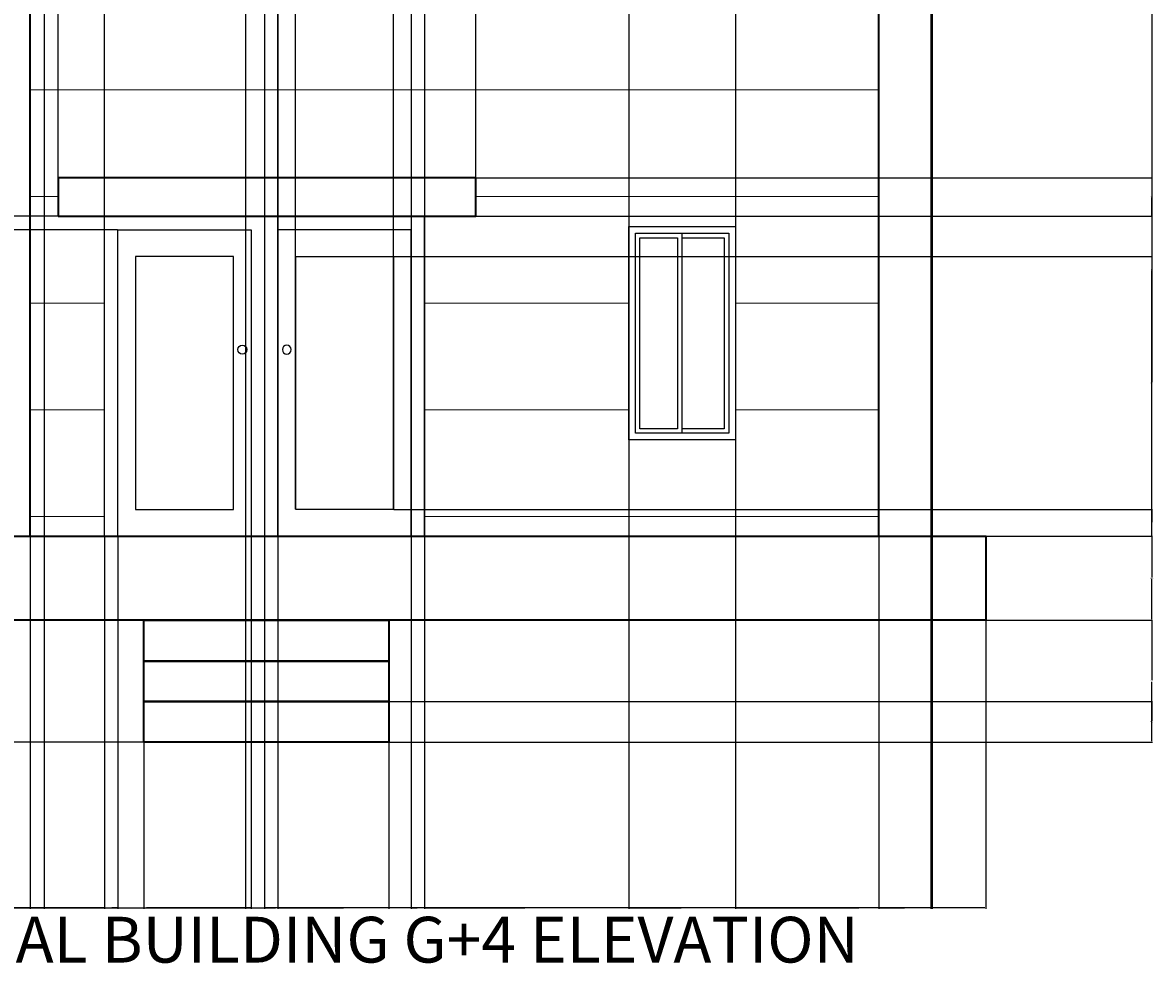
# Model space of a CAD drawing. Units: inches. Extents: x 10 to 404, y -77 to 696.
# Tile 2 of 5: x 149 to 404, y -77 to 135. Entities that reach past the tile are written whole.
import ezdxf

# ---------------------------------------------------------------- set-up
doc = ezdxf.new("R2010")
doc.units = ezdxf.units.IN
doc.header["$MEASUREMENT"] = 0
for name, color, linetype, lineweight in [('A-ANNO-DIMS', 2, 'Continuous', 18), ('A-ANNO-TEXT', 7, 'Continuous', 25), ('A-DOOR', 4, 'Continuous', 25), ('A-ELEV', 7, 'Continuous', 35), ('A-ELEV-PATT', 8, 'Continuous', 13), ('A-GLAZ', 4, 'Continuous', 25)]:
    doc.layers.add(name, color=color, linetype=linetype, lineweight=lineweight)
doc.styles.get("Standard").update_dxf_attribs({"font": 'arial.ttf'})
doc.dimstyles.get("Standard").update_dxf_attribs({"dimtxt": 0.18, "dimasz": 0.18, "dimexe": 0.18, "dimexo": 0.0625, "dimgap": 0.09, "dimtad": 0, "dimtih": 1, "dimtoh": 1, "dimdec": 4, "dimzin": 0, "dimdsep": 46, "dimtxsty": 'Standard', "dimcen": 0.09, "dimadec": 0, "dimazin": 0, "dimtfac": 1, "dimtdec": 4, "dimtofl": 0, "dimtmove": 0, "dimatfit": 3, "dimfxl": 1, "dimtolj": 1, "dimtzin": 0, "dimarcsym": 0})

# ---------------------------------------------------------------- blocks, each defined once
blk = doc.blocks.new('*U4')
blk.add_lwpolyline([(3.12, 0.01), (0.12, 0.01), (0.12, 72.01), (36.12, 72.01), (36.12, 0.01), (33.12, 0.01)])
for points in [[(33.12, 68.99), (33.12, 0.01), (3.12, 0.01), (3.12, 68.99)], [(29.12, 6.01), (29.12, 62.99), (7.12, 62.99), (7.12, 6.01)]]:
    blk.add_lwpolyline(points, close=True)
blk.add_circle((31.12, 42.01), 1)
blk = doc.blocks.new('*U5')
for p, q in [((1.5, 1.5), (1.5, 46.5)), ((1.5, 46.5), (12, 46.5)), ((12, 1.5), (12, 46.5)), ((12, 46.5), (22.5, 46.5)), ((22.5, 46.5), (22.5, 1.5)), ((12, 1.5), (1.5, 1.5)), ((22.5, 1.5), (12, 1.5))]:
    blk.add_line(p, q)
blk.add_lwpolyline([(0, 0), (0, 48), (24, 48), (24, 0)], close=True)
for points in [[(11, 45.5), (11, 2.5), (2.5, 2.5), (2.5, 45.5), (11, 45.5)], [(12, 45.5), (21.5, 45.5), (21.5, 2.5), (12, 2.5)]]:
    blk.add_lwpolyline(points)
blk = doc.blocks.new('*D9')
at = {"layer": 'A-ANNO-DIMS', "color": 0, "lineweight": -2, "transparency": 16777216}
for p, q in [((47.29, 0.6), (47.29, -64.31)), ((365.94, 0.6), (365.94, -64.31)), ((47.47, -64.13), (206.15, -64.13)), ((365.76, -64.13), (207.08, -64.13))]:
    blk.add_line(p, q, dxfattribs=at)
at = {"layer": 'A-ANNO-DIMS', "color": 0, "transparency": 16777216}
for points in [[(47.47, -64.1), (47.47, -64.16), (47.29, -64.13)], [(365.76, -64.1), (365.76, -64.16), (365.94, -64.13)]]:
    blk.add_solid(points, dxfattribs=at)
at = {"layer": 'Defpoints', "color": 0, "transparency": 16777216}
for p in [(47.29, 0.67), (365.94, 0.67), (365.94, -64.13)]:
    blk.add_point(p, dxfattribs=at)
at = {"layer": 'A-ANNO-DIMS', "color": 0, "transparency": 16777216, "insert": (206.61, -64.13), "char_height": 0.18, "attachment_point": 5}
blk.add_mtext('\\A1;318.65', dxfattribs=at)
blk = doc.blocks.new('*D10')
at = {"layer": 'A-ANNO-DIMS', "color": 0, "lineweight": -2, "transparency": 16777216}
for p, q in [((65.94, 657.96), (9.76, 657.96)), ((9.94, 657.78), (9.94, 315.77)), ((9.94, -26.6), (9.94, 315.41)), ((176.46, -26.78), (9.76, -26.78))]:
    blk.add_line(p, q, dxfattribs=at)
at = {"layer": 'A-ANNO-DIMS', "color": 0, "transparency": 16777216}
for points in [[(9.91, 657.78), (9.97, 657.78), (9.94, 657.96)], [(9.91, -26.6), (9.97, -26.6), (9.94, -26.78)]]:
    blk.add_solid(points, dxfattribs=at)
at = {"layer": 'Defpoints', "color": 0, "transparency": 16777216}
for p in [(9.94, 657.96), (66.01, 657.96), (176.53, -26.78)]:
    blk.add_point(p, dxfattribs=at)
at = {"layer": 'A-ANNO-DIMS', "color": 0, "transparency": 16777216, "insert": (9.94, 315.59), "char_height": 0.18, "attachment_point": 5}
blk.add_mtext('\\A1;684.7', dxfattribs=at)
blk = doc.blocks.new('*D13')
at = {"layer": 'A-ANNO-DIMS', "color": 0, "lineweight": -2, "transparency": 16777216}
for p, q in [((81.51, 19.49), (81.51, -64.31)), ((167.67, 19.49), (167.67, -64.31)), ((81.69, -64.13), (124.19, -64.13)), ((167.49, -64.13), (124.98, -64.13))]:
    blk.add_line(p, q, dxfattribs=at)
at = {"layer": 'A-ANNO-DIMS', "color": 0, "transparency": 16777216}
for points in [[(81.69, -64.1), (81.69, -64.16), (81.51, -64.13)], [(167.49, -64.1), (167.49, -64.16), (167.67, -64.13)]]:
    blk.add_solid(points, dxfattribs=at)
at = {"layer": 'Defpoints', "color": 0, "transparency": 16777216}
for p in [(81.51, 19.55), (167.67, 19.55), (167.67, -64.13)]:
    blk.add_point(p, dxfattribs=at)
at = {"layer": 'A-ANNO-DIMS', "color": 0, "transparency": 16777216, "insert": (124.59, -64.13), "char_height": 0.18, "attachment_point": 5}
blk.add_mtext('\\A1;86.16', dxfattribs=at)
blk = doc.blocks.new('*D14')
at = {"layer": 'A-ANNO-DIMS', "color": 0, "lineweight": -2, "transparency": 16777216}
for p, q in [((285.62, 41.17), (285.62, -64.31)), ((239.67, 19.49), (239.67, -64.31)), ((239.85, -64.13), (262.25, -64.13)), ((285.44, -64.13), (263.04, -64.13))]:
    blk.add_line(p, q, dxfattribs=at)
at = {"layer": 'A-ANNO-DIMS', "color": 0, "transparency": 16777216}
for points in [[(239.85, -64.1), (239.85, -64.16), (239.67, -64.13)], [(285.44, -64.1), (285.44, -64.16), (285.62, -64.13)]]:
    blk.add_solid(points, dxfattribs=at)
at = {"layer": 'Defpoints', "color": 0, "transparency": 16777216}
for p in [(285.62, 41.23), (239.67, 19.55), (285.62, -64.13)]:
    blk.add_point(p, dxfattribs=at)
at = {"layer": 'A-ANNO-DIMS', "color": 0, "transparency": 16777216, "insert": (262.64, -64.13), "char_height": 0.18, "attachment_point": 5}
blk.add_mtext('\\A1;45.95', dxfattribs=at)
blk = doc.blocks.new('*D15')
at = {"layer": 'A-ANNO-DIMS', "color": 0, "lineweight": -2, "transparency": 16777216}
for p, q in [((285.62, 41.17), (285.62, -64.31)), ((309.62, 41.17), (309.62, -64.31)), ((285.8, -64.13), (297.4, -64.13)), ((309.44, -64.13), (297.84, -64.13))]:
    blk.add_line(p, q, dxfattribs=at)
at = {"layer": 'A-ANNO-DIMS', "color": 0, "transparency": 16777216}
for points in [[(285.8, -64.1), (285.8, -64.16), (285.62, -64.13)], [(309.44, -64.1), (309.44, -64.16), (309.62, -64.13)]]:
    blk.add_solid(points, dxfattribs=at)
at = {"layer": 'Defpoints', "color": 0, "transparency": 16777216}
for p in [(285.62, 41.23), (309.62, 41.23), (309.62, -64.13)]:
    blk.add_point(p, dxfattribs=at)
at = {"layer": 'A-ANNO-DIMS', "color": 0, "transparency": 16777216, "insert": (297.62, -64.13), "char_height": 0.18, "attachment_point": 5}
blk.add_mtext('\\A1;24', dxfattribs=at)
blk = doc.blocks.new('*D16')
at = {"layer": 'A-ANNO-DIMS', "color": 0, "lineweight": -2, "transparency": 16777216}
for p, q in [((309.62, 41.17), (309.62, -64.31)), ((365.94, 0.6), (365.94, -64.31)), ((309.8, -64.13), (337.38, -64.13)), ((365.76, -64.13), (338.17, -64.13))]:
    blk.add_line(p, q, dxfattribs=at)
at = {"layer": 'A-ANNO-DIMS', "color": 0, "transparency": 16777216}
for points in [[(309.8, -64.1), (309.8, -64.16), (309.62, -64.13)], [(365.76, -64.1), (365.76, -64.16), (365.94, -64.13)]]:
    blk.add_solid(points, dxfattribs=at)
at = {"layer": 'Defpoints', "color": 0, "transparency": 16777216}
for p in [(309.62, 41.23), (365.94, 0.67), (365.94, -64.13)]:
    blk.add_point(p, dxfattribs=at)
at = {"layer": 'A-ANNO-DIMS', "color": 0, "transparency": 16777216, "insert": (337.78, -64.13), "char_height": 0.18, "attachment_point": 5}
blk.add_mtext('\\A1;56.32', dxfattribs=at)
blk = doc.blocks.new('*D23')
at = {"layer": 'A-ANNO-DIMS', "color": 0, "lineweight": -2, "transparency": 16777216}
for p, q in [((341.87, 355.52), (341.87, -64.31)), ((353.59, 355.52), (353.59, -64.31)), ((342.05, -64.13), (347.27, -64.13)), ((353.41, -64.13), (348.18, -64.13))]:
    blk.add_line(p, q, dxfattribs=at)
at = {"layer": 'A-ANNO-DIMS', "color": 0, "transparency": 16777216}
for points in [[(342.05, -64.1), (342.05, -64.16), (341.87, -64.13)], [(353.41, -64.1), (353.41, -64.16), (353.59, -64.13)]]:
    blk.add_solid(points, dxfattribs=at)
at = {"layer": 'Defpoints', "color": 0, "transparency": 16777216}
for p in [(341.87, 355.58), (353.59, 355.58), (353.59, -64.13)]:
    blk.add_point(p, dxfattribs=at)
at = {"layer": 'A-ANNO-DIMS', "color": 0, "transparency": 16777216, "insert": (347.73, -64.13), "char_height": 0.18, "attachment_point": 5}
blk.add_mtext('\\A1;11.723', dxfattribs=at)
blk = doc.blocks.new('*D24')
at = {"layer": 'A-ANNO-DIMS', "color": 0, "lineweight": -2, "transparency": 16777216}
for p, q in [((176.53, -26.84), (176.53, -64.31)), ((231.66, -26.84), (231.66, -64.31)), ((176.71, -64.13), (203.7, -64.13)), ((231.48, -64.13), (204.49, -64.13))]:
    blk.add_line(p, q, dxfattribs=at)
at = {"layer": 'A-ANNO-DIMS', "color": 0, "transparency": 16777216}
for points in [[(176.71, -64.1), (176.71, -64.16), (176.53, -64.13)], [(231.48, -64.1), (231.48, -64.16), (231.66, -64.13)]]:
    blk.add_solid(points, dxfattribs=at)
at = {"layer": 'Defpoints', "color": 0, "transparency": 16777216}
for p in [(176.53, -26.78), (231.66, -26.78), (231.66, -64.13)]:
    blk.add_point(p, dxfattribs=at)
at = {"layer": 'A-ANNO-DIMS', "color": 0, "transparency": 16777216, "insert": (204.09, -64.13), "char_height": 0.18, "attachment_point": 5}
blk.add_mtext('\\A1;55.13', dxfattribs=at)
blk = doc.blocks.new('*D25')
at = {"layer": 'A-ANNO-DIMS', "color": 0, "lineweight": -2, "transparency": 16777216}
for p, q in [((231.72, 0.67), (403.47, 0.67)), ((403.29, 0.49), (403.29, -12.88)), ((403.29, -26.6), (403.29, -13.24)), ((231.72, -26.78), (403.47, -26.78))]:
    blk.add_line(p, q, dxfattribs=at)
at = {"layer": 'A-ANNO-DIMS', "color": 0, "transparency": 16777216}
for points in [[(403.26, 0.49), (403.32, 0.49), (403.29, 0.67)], [(403.26, -26.6), (403.32, -26.6), (403.29, -26.78)]]:
    blk.add_solid(points, dxfattribs=at)
at = {"layer": 'Defpoints', "color": 0, "transparency": 16777216}
for p in [(231.66, 0.67), (231.66, -26.78), (403.29, -26.78)]:
    blk.add_point(p, dxfattribs=at)
at = {"layer": 'A-ANNO-DIMS', "color": 0, "transparency": 16777216, "insert": (403.29, -13.06), "char_height": 0.18, "attachment_point": 5}
blk.add_mtext('\\A1;27.45', dxfattribs=at)
blk = doc.blocks.new('*D26')
at = {"layer": 'A-ANNO-DIMS', "color": 0, "lineweight": -2, "transparency": 16777216}
for p, q in [((231.72, -17.67), (403.47, -17.67)), ((403.29, -17.85), (403.29, -22.04)), ((403.29, -26.6), (403.29, -22.41)), ((231.72, -26.78), (403.47, -26.78))]:
    blk.add_line(p, q, dxfattribs=at)
at = {"layer": 'A-ANNO-DIMS', "color": 0, "transparency": 16777216}
for points in [[(403.26, -17.85), (403.32, -17.85), (403.29, -17.67)], [(403.26, -26.6), (403.32, -26.6), (403.29, -26.78)]]:
    blk.add_solid(points, dxfattribs=at)
at = {"layer": 'Defpoints', "color": 0, "transparency": 16777216}
for p in [(231.66, -17.67), (231.66, -26.78), (403.29, -26.78)]:
    blk.add_point(p, dxfattribs=at)
at = {"layer": 'A-ANNO-DIMS', "color": 0, "transparency": 16777216, "insert": (403.29, -22.22), "char_height": 0.18, "attachment_point": 5}
blk.add_mtext('\\A1;9.115', dxfattribs=at)
blk = doc.blocks.new('*D27')
at = {"layer": 'A-ANNO-DIMS', "color": 0, "lineweight": -2, "transparency": 16777216}
for p, q in [((366, 19.55), (403.47, 19.55)), ((403.29, 19.37), (403.29, 10.29)), ((403.29, 0.85), (403.29, 9.93)), ((366, 0.67), (403.47, 0.67))]:
    blk.add_line(p, q, dxfattribs=at)
at = {"layer": 'A-ANNO-DIMS', "color": 0, "transparency": 16777216}
for points in [[(403.26, 19.37), (403.32, 19.37), (403.29, 19.55)], [(403.26, 0.85), (403.32, 0.85), (403.29, 0.67)]]:
    blk.add_solid(points, dxfattribs=at)
at = {"layer": 'Defpoints', "color": 0, "transparency": 16777216}
for p in [(365.94, 19.55), (403.29, 19.55), (365.94, 0.67)]:
    blk.add_point(p, dxfattribs=at)
at = {"layer": 'A-ANNO-DIMS', "color": 0, "transparency": 16777216, "insert": (403.29, 10.11), "char_height": 0.18, "attachment_point": 5}
blk.add_mtext('\\A1;18.887', dxfattribs=at)
blk = doc.blocks.new('*D28')
at = {"layer": 'A-ANNO-DIMS', "color": 0, "lineweight": -2, "transparency": 16777216}
for p, q in [((341.93, 139.55), (403.47, 139.55)), ((403.29, 139.37), (403.29, 79.74)), ((403.29, 19.73), (403.29, 79.37)), ((341.93, 19.55), (403.47, 19.55))]:
    blk.add_line(p, q, dxfattribs=at)
at = {"layer": 'A-ANNO-DIMS', "color": 0, "transparency": 16777216}
for points in [[(403.26, 139.37), (403.32, 139.37), (403.29, 139.55)], [(403.26, 19.73), (403.32, 19.73), (403.29, 19.55)]]:
    blk.add_solid(points, dxfattribs=at)
at = {"layer": 'Defpoints', "color": 0, "transparency": 16777216}
for p in [(341.87, 139.55), (403.29, 139.55), (341.87, 19.55)]:
    blk.add_point(p, dxfattribs=at)
at = {"layer": 'A-ANNO-DIMS', "color": 0, "transparency": 16777216, "insert": (403.29, 79.55), "char_height": 0.18, "attachment_point": 5}
blk.add_mtext('\\A1;120', dxfattribs=at)
blk = doc.blocks.new('*D39')
at = {"layer": 'A-ANNO-DIMS', "color": 0, "lineweight": -2, "transparency": 16777216}
for p, q in [((341.87, 259.49), (341.87, -64.31)), ((353.87, 259.49), (353.87, -64.31)), ((342.05, -64.13), (347.66, -64.13)), ((353.69, -64.13), (348.08, -64.13))]:
    blk.add_line(p, q, dxfattribs=at)
at = {"layer": 'A-ANNO-DIMS', "color": 0, "transparency": 16777216}
for points in [[(342.05, -64.1), (342.05, -64.16), (341.87, -64.13)], [(353.69, -64.1), (353.69, -64.16), (353.87, -64.13)]]:
    blk.add_solid(points, dxfattribs=at)
at = {"layer": 'Defpoints', "color": 0, "transparency": 16777216}
for p in [(341.87, 259.55), (353.87, 259.55), (353.87, -64.13)]:
    blk.add_point(p, dxfattribs=at)
at = {"layer": 'A-ANNO-DIMS', "color": 0, "transparency": 16777216, "insert": (347.87, -64.13), "char_height": 0.18, "attachment_point": 5}
blk.add_mtext('\\A1;12', dxfattribs=at)
blk = doc.blocks.new('*D42')
at = {"layer": 'A-ANNO-DIMS', "color": 0, "lineweight": -2, "transparency": 16777216}
for p, q in [((150.93, 259.49), (150.93, -64.31)), ((154.06, 142.19), (154.06, -64.31)), ((151.11, -64.13), (152.17, -64.13)), ((153.88, -64.13), (152.82, -64.13))]:
    blk.add_line(p, q, dxfattribs=at)
at = {"layer": 'A-ANNO-DIMS', "color": 0, "transparency": 16777216}
for points in [[(151.11, -64.1), (151.11, -64.16), (150.93, -64.13)], [(153.88, -64.1), (153.88, -64.16), (154.06, -64.13)]]:
    blk.add_solid(points, dxfattribs=at)
at = {"layer": 'Defpoints', "color": 0, "transparency": 16777216}
for p in [(150.93, 259.55), (154.06, 142.25), (154.06, -64.13)]:
    blk.add_point(p, dxfattribs=at)
at = {"layer": 'A-ANNO-DIMS', "color": 0, "transparency": 16777216, "insert": (152.5, -64.13), "char_height": 0.18, "attachment_point": 5}
blk.add_mtext('\\A1;3.13', dxfattribs=at)
blk = doc.blocks.new('*D43')
at = {"layer": 'A-ANNO-DIMS', "color": 0, "lineweight": -2, "transparency": 16777216}
for p, q in [((154.06, 142.19), (154.06, -64.31)), ((199.39, 142.19), (199.39, -64.31)), ((154.24, -64.13), (176.33, -64.13)), ((199.21, -64.13), (177.13, -64.13))]:
    blk.add_line(p, q, dxfattribs=at)
at = {"layer": 'A-ANNO-DIMS', "color": 0, "transparency": 16777216}
for points in [[(154.24, -64.1), (154.24, -64.16), (154.06, -64.13)], [(199.21, -64.1), (199.21, -64.16), (199.39, -64.13)]]:
    blk.add_solid(points, dxfattribs=at)
at = {"layer": 'Defpoints', "color": 0, "transparency": 16777216}
for p in [(154.06, 142.25), (199.39, 142.25), (199.39, -64.13)]:
    blk.add_point(p, dxfattribs=at)
at = {"layer": 'A-ANNO-DIMS', "color": 0, "transparency": 16777216, "insert": (176.73, -64.13), "char_height": 0.18, "attachment_point": 5}
blk.add_mtext('\\A1;45.33', dxfattribs=at)
blk = doc.blocks.new('*D48')
at = {"layer": 'A-ANNO-DIMS', "color": 0, "lineweight": -2, "transparency": 16777216}
for p, q in [((285.62, 521.17), (285.62, -64.31)), ((239.67, 499.54), (239.67, -64.31)), ((239.85, -64.13), (262.25, -64.13)), ((285.44, -64.13), (263.04, -64.13))]:
    blk.add_line(p, q, dxfattribs=at)
at = {"layer": 'A-ANNO-DIMS', "color": 0, "transparency": 16777216}
for points in [[(239.85, -64.1), (239.85, -64.16), (239.67, -64.13)], [(285.44, -64.1), (285.44, -64.16), (285.62, -64.13)]]:
    blk.add_solid(points, dxfattribs=at)
at = {"layer": 'Defpoints', "color": 0, "transparency": 16777216}
for p in [(285.62, 521.23), (239.67, 499.6), (285.62, -64.13)]:
    blk.add_point(p, dxfattribs=at)
at = {"layer": 'A-ANNO-DIMS', "color": 0, "transparency": 16777216, "insert": (262.64, -64.13), "char_height": 0.18, "attachment_point": 5}
blk.add_mtext('\\A1;45.95', dxfattribs=at)
blk = doc.blocks.new('*D49')
at = {"layer": 'A-ANNO-DIMS', "color": 0, "lineweight": -2, "transparency": 16777216}
for p, q in [((285.62, 521.17), (285.62, -64.31)), ((309.62, 521.17), (309.62, -64.31)), ((285.8, -64.13), (297.4, -64.13)), ((309.44, -64.13), (297.84, -64.13))]:
    blk.add_line(p, q, dxfattribs=at)
at = {"layer": 'A-ANNO-DIMS', "color": 0, "transparency": 16777216}
for points in [[(285.8, -64.1), (285.8, -64.16), (285.62, -64.13)], [(309.44, -64.1), (309.44, -64.16), (309.62, -64.13)]]:
    blk.add_solid(points, dxfattribs=at)
at = {"layer": 'Defpoints', "color": 0, "transparency": 16777216}
for p in [(285.62, 521.23), (309.62, 521.23), (309.62, -64.13)]:
    blk.add_point(p, dxfattribs=at)
at = {"layer": 'A-ANNO-DIMS', "color": 0, "transparency": 16777216, "insert": (297.62, -64.13), "char_height": 0.18, "attachment_point": 5}
blk.add_mtext('\\A1;24', dxfattribs=at)
blk = doc.blocks.new('*D50')
at = {"layer": 'A-ANNO-DIMS', "color": 0, "lineweight": -2, "transparency": 16777216}
for p, q in [((157.2, 100.31), (157.2, 695.87)), ((157.38, 695.69), (161.98, 695.69)), ((167.49, 695.69), (162.89, 695.69)), ((167.67, 91.62), (167.67, 695.87))]:
    blk.add_line(p, q, dxfattribs=at)
at = {"layer": 'A-ANNO-DIMS', "color": 0, "transparency": 16777216}
for points in [[(157.38, 695.72), (157.38, 695.66), (157.2, 695.69)], [(167.49, 695.72), (167.49, 695.66), (167.67, 695.69)]]:
    blk.add_solid(points, dxfattribs=at)
at = {"layer": 'Defpoints', "color": 0, "transparency": 16777216}
for p in [(167.67, 695.69), (157.2, 100.24), (167.67, 91.55)]:
    blk.add_point(p, dxfattribs=at)
at = {"layer": 'A-ANNO-DIMS', "color": 0, "transparency": 16777216, "insert": (162.43, 695.69), "char_height": 0.18, "attachment_point": 5}
blk.add_mtext('\\A1;10.469', dxfattribs=at)
blk = doc.blocks.new('*D51')
at = {"layer": 'A-ANNO-DIMS', "color": 0, "lineweight": -2, "transparency": 16777216}
for p, q in [((167.67, 91.62), (167.67, 695.87)), ((167.85, 695.69), (209.06, 695.69)), ((251.06, 695.69), (209.85, 695.69)), ((251.24, 100.31), (251.24, 695.87))]:
    blk.add_line(p, q, dxfattribs=at)
at = {"layer": 'A-ANNO-DIMS', "color": 0, "transparency": 16777216}
for points in [[(167.85, 695.72), (167.85, 695.66), (167.67, 695.69)], [(251.06, 695.72), (251.06, 695.66), (251.24, 695.69)]]:
    blk.add_solid(points, dxfattribs=at)
at = {"layer": 'Defpoints', "color": 0, "transparency": 16777216}
for p in [(251.24, 695.69), (251.24, 100.24), (167.67, 91.55)]:
    blk.add_point(p, dxfattribs=at)
at = {"layer": 'A-ANNO-DIMS', "color": 0, "transparency": 16777216, "insert": (209.45, 695.69), "char_height": 0.18, "attachment_point": 5}
blk.add_mtext('\\A1;83.57', dxfattribs=at)
blk = doc.blocks.new('*D52')
at = {"layer": 'A-ANNO-DIMS', "color": 0, "lineweight": -2, "transparency": 16777216}
for p, q in [((251.3, 100.24), (403.47, 100.24)), ((403.29, 100.06), (403.29, 96.08)), ((403.29, 91.73), (403.29, 95.72)), ((251.3, 91.55), (403.47, 91.55))]:
    blk.add_line(p, q, dxfattribs=at)
at = {"layer": 'A-ANNO-DIMS', "color": 0, "transparency": 16777216}
for points in [[(403.26, 100.06), (403.32, 100.06), (403.29, 100.24)], [(403.26, 91.73), (403.32, 91.73), (403.29, 91.55)]]:
    blk.add_solid(points, dxfattribs=at)
at = {"layer": 'Defpoints', "color": 0, "transparency": 16777216}
for p in [(251.24, 100.24), (403.29, 100.24), (251.24, 91.55)]:
    blk.add_point(p, dxfattribs=at)
at = {"layer": 'A-ANNO-DIMS', "color": 0, "transparency": 16777216, "insert": (403.29, 95.9), "char_height": 0.18, "attachment_point": 5}
blk.add_mtext('\\A1;8.69', dxfattribs=at)
blk = doc.blocks.new('*D53')
at = {"layer": 'A-ANNO-DIMS', "color": 0, "lineweight": -2, "transparency": 16777216}
for p, q in [((251.3, 91.55), (403.47, 91.55)), ((403.29, 91.37), (403.29, 55.73)), ((403.29, 19.73), (403.29, 55.37)), ((239.73, 19.55), (403.47, 19.55))]:
    blk.add_line(p, q, dxfattribs=at)
at = {"layer": 'A-ANNO-DIMS', "color": 0, "transparency": 16777216}
for points in [[(403.26, 91.37), (403.32, 91.37), (403.29, 91.55)], [(403.26, 19.73), (403.32, 19.73), (403.29, 19.55)]]:
    blk.add_solid(points, dxfattribs=at)
at = {"layer": 'Defpoints', "color": 0, "transparency": 16777216}
for p in [(251.24, 91.55), (403.29, 91.55), (239.67, 19.55)]:
    blk.add_point(p, dxfattribs=at)
at = {"layer": 'A-ANNO-DIMS', "color": 0, "transparency": 16777216, "insert": (403.29, 55.55), "char_height": 0.18, "attachment_point": 5}
blk.add_mtext('\\A1;72', dxfattribs=at)
blk = doc.blocks.new('*D54')
at = {"layer": 'A-ANNO-DIMS', "color": 0, "lineweight": -2, "transparency": 16777216}
for p, q in [((167.6, 91.55), (9.76, 91.55)), ((9.94, 91.37), (9.94, 55.73)), ((9.94, 19.73), (9.94, 55.37)), ((167.6, 19.55), (9.76, 19.55))]:
    blk.add_line(p, q, dxfattribs=at)
at = {"layer": 'A-ANNO-DIMS', "color": 0, "transparency": 16777216}
for points in [[(9.91, 91.37), (9.97, 91.37), (9.94, 91.55)], [(9.91, 19.73), (9.97, 19.73), (9.94, 19.55)]]:
    blk.add_solid(points, dxfattribs=at)
at = {"layer": 'Defpoints', "color": 0, "transparency": 16777216}
for p in [(9.94, 91.55), (167.67, 91.55), (167.67, 19.55)]:
    blk.add_point(p, dxfattribs=at)
at = {"layer": 'A-ANNO-DIMS', "color": 0, "transparency": 16777216, "insert": (9.94, 55.55), "char_height": 0.18, "attachment_point": 5}
blk.add_mtext('\\A1;72', dxfattribs=at)
blk = doc.blocks.new('*D55')
at = {"layer": 'A-ANNO-DIMS', "color": 0, "lineweight": -2, "transparency": 16777216}
for p, q in [((170.6, 88.53), (9.76, 88.53)), ((9.94, 88.35), (9.94, 54.22)), ((9.94, 19.73), (9.94, 53.86)), ((170.6, 19.55), (9.76, 19.55))]:
    blk.add_line(p, q, dxfattribs=at)
at = {"layer": 'A-ANNO-DIMS', "color": 0, "transparency": 16777216}
for points in [[(9.91, 88.35), (9.97, 88.35), (9.94, 88.53)], [(9.91, 19.73), (9.97, 19.73), (9.94, 19.55)]]:
    blk.add_solid(points, dxfattribs=at)
at = {"layer": 'Defpoints', "color": 0, "transparency": 16777216}
for p in [(9.94, 88.53), (170.67, 88.53), (170.67, 19.55)]:
    blk.add_point(p, dxfattribs=at)
at = {"layer": 'A-ANNO-DIMS', "color": 0, "transparency": 16777216, "insert": (9.94, 54.04), "char_height": 0.18, "attachment_point": 5}
blk.add_mtext('\\A1;68.98', dxfattribs=at)
blk = doc.blocks.new('*D56')
at = {"layer": 'A-ANNO-DIMS', "color": 0, "lineweight": -2, "transparency": 16777216}
for p, q in [((167.67, 19.49), (167.67, -64.31)), ((170.67, 19.49), (170.67, -64.31)), ((167.85, -64.13), (169.02, -64.13)), ((170.49, -64.13), (169.32, -64.13))]:
    blk.add_line(p, q, dxfattribs=at)
at = {"layer": 'A-ANNO-DIMS', "color": 0, "transparency": 16777216}
for points in [[(167.85, -64.1), (167.85, -64.16), (167.67, -64.13)], [(170.49, -64.1), (170.49, -64.16), (170.67, -64.13)]]:
    blk.add_solid(points, dxfattribs=at)
at = {"layer": 'Defpoints', "color": 0, "transparency": 16777216}
for p in [(167.67, 19.55), (170.67, 19.55), (170.67, -64.13)]:
    blk.add_point(p, dxfattribs=at)
at = {"layer": 'A-ANNO-DIMS', "color": 0, "transparency": 16777216, "insert": (169.17, -64.13), "char_height": 0.18, "attachment_point": 5}
blk.add_mtext('\\A1;3', dxfattribs=at)
blk = doc.blocks.new('*D57')
at = {"layer": 'A-ANNO-DIMS', "color": 0, "lineweight": -2, "transparency": 16777216}
for p, q in [((170.67, 19.49), (170.67, -64.31)), ((200.67, 19.49), (200.67, -64.31)), ((170.85, -64.13), (185.45, -64.13)), ((200.49, -64.13), (185.89, -64.13))]:
    blk.add_line(p, q, dxfattribs=at)
at = {"layer": 'A-ANNO-DIMS', "color": 0, "transparency": 16777216}
for points in [[(170.85, -64.1), (170.85, -64.16), (170.67, -64.13)], [(200.49, -64.1), (200.49, -64.16), (200.67, -64.13)]]:
    blk.add_solid(points, dxfattribs=at)
at = {"layer": 'Defpoints', "color": 0, "transparency": 16777216}
for p in [(170.67, 19.55), (200.67, 19.55), (200.67, -64.13)]:
    blk.add_point(p, dxfattribs=at)
at = {"layer": 'A-ANNO-DIMS', "color": 0, "transparency": 16777216, "insert": (185.67, -64.13), "char_height": 0.18, "attachment_point": 5}
blk.add_mtext('\\A1;30', dxfattribs=at)
blk = doc.blocks.new('*D58')
at = {"layer": 'A-ANNO-DIMS', "color": 0, "lineweight": -2, "transparency": 16777216}
for p, q in [((200.67, 19.49), (200.67, -64.31)), ((206.67, 19.49), (206.67, -64.31)), ((200.85, -64.13), (203.52, -64.13)), ((206.49, -64.13), (203.82, -64.13))]:
    blk.add_line(p, q, dxfattribs=at)
at = {"layer": 'A-ANNO-DIMS', "color": 0, "transparency": 16777216}
for points in [[(200.85, -64.1), (200.85, -64.16), (200.67, -64.13)], [(206.49, -64.1), (206.49, -64.16), (206.67, -64.13)]]:
    blk.add_solid(points, dxfattribs=at)
at = {"layer": 'Defpoints', "color": 0, "transparency": 16777216}
for p in [(200.67, 19.55), (206.67, 19.55), (206.67, -64.13)]:
    blk.add_point(p, dxfattribs=at)
at = {"layer": 'A-ANNO-DIMS', "color": 0, "transparency": 16777216, "insert": (203.67, -64.13), "char_height": 0.18, "attachment_point": 5}
blk.add_mtext('\\A1;6', dxfattribs=at)
blk = doc.blocks.new('*D59')
at = {"layer": 'A-ANNO-DIMS', "color": 0, "lineweight": -2, "transparency": 16777216}
for p, q in [((206.67, 19.49), (206.67, -64.31)), ((236.67, 19.49), (236.67, -64.31)), ((206.85, -64.13), (221.45, -64.13)), ((236.49, -64.13), (221.89, -64.13))]:
    blk.add_line(p, q, dxfattribs=at)
at = {"layer": 'A-ANNO-DIMS', "color": 0, "transparency": 16777216}
for points in [[(206.85, -64.1), (206.85, -64.16), (206.67, -64.13)], [(236.49, -64.1), (236.49, -64.16), (236.67, -64.13)]]:
    blk.add_solid(points, dxfattribs=at)
at = {"layer": 'Defpoints', "color": 0, "transparency": 16777216}
for p in [(206.67, 19.55), (236.67, 19.55), (236.67, -64.13)]:
    blk.add_point(p, dxfattribs=at)
at = {"layer": 'A-ANNO-DIMS', "color": 0, "transparency": 16777216, "insert": (221.67, -64.13), "char_height": 0.18, "attachment_point": 5}
blk.add_mtext('\\A1;30', dxfattribs=at)
blk = doc.blocks.new('*D60')
at = {"layer": 'A-ANNO-DIMS', "color": 0, "lineweight": -2, "transparency": 16777216}
for p, q in [((236.67, 19.49), (236.67, -64.31)), ((239.67, 19.49), (239.67, -64.31)), ((236.85, -64.13), (238.02, -64.13)), ((239.49, -64.13), (238.32, -64.13))]:
    blk.add_line(p, q, dxfattribs=at)
at = {"layer": 'A-ANNO-DIMS', "color": 0, "transparency": 16777216}
for points in [[(236.85, -64.1), (236.85, -64.16), (236.67, -64.13)], [(239.49, -64.1), (239.49, -64.16), (239.67, -64.13)]]:
    blk.add_solid(points, dxfattribs=at)
at = {"layer": 'Defpoints', "color": 0, "transparency": 16777216}
for p in [(236.67, 19.55), (239.67, 19.55), (239.67, -64.13)]:
    blk.add_point(p, dxfattribs=at)
at = {"layer": 'A-ANNO-DIMS', "color": 0, "transparency": 16777216, "insert": (238.17, -64.13), "char_height": 0.18, "attachment_point": 5}
blk.add_mtext('\\A1;3', dxfattribs=at)
blk = doc.blocks.new('*D61')
at = {"layer": 'A-ANNO-DIMS', "color": 0, "lineweight": -2, "transparency": 16777216}
for p, q in [((206.67, 19.62), (206.67, 695.87)), ((206.85, 695.69), (208.51, 695.69)), ((210.49, 695.69), (208.82, 695.69)), ((210.67, 25.62), (210.67, 695.87))]:
    blk.add_line(p, q, dxfattribs=at)
at = {"layer": 'A-ANNO-DIMS', "color": 0, "transparency": 16777216}
for points in [[(206.85, 695.72), (206.85, 695.66), (206.67, 695.69)], [(210.49, 695.72), (210.49, 695.66), (210.67, 695.69)]]:
    blk.add_solid(points, dxfattribs=at)
at = {"layer": 'Defpoints', "color": 0, "transparency": 16777216}
for p in [(210.67, 695.69), (210.67, 25.55), (206.67, 19.55)]:
    blk.add_point(p, dxfattribs=at)
at = {"layer": 'A-ANNO-DIMS', "color": 0, "transparency": 16777216, "insert": (208.67, 695.69), "char_height": 0.18, "attachment_point": 5}
blk.add_mtext('\\A1;4', dxfattribs=at)
blk = doc.blocks.new('*D62')
at = {"layer": 'A-ANNO-DIMS', "color": 0, "lineweight": -2, "transparency": 16777216}
for p, q in [((210.67, 25.62), (210.67, 695.87)), ((210.85, 695.69), (221.45, 695.69)), ((232.49, 695.69), (221.89, 695.69)), ((232.67, 25.62), (232.67, 695.87))]:
    blk.add_line(p, q, dxfattribs=at)
at = {"layer": 'A-ANNO-DIMS', "color": 0, "transparency": 16777216}
for points in [[(210.85, 695.72), (210.85, 695.66), (210.67, 695.69)], [(232.49, 695.72), (232.49, 695.66), (232.67, 695.69)]]:
    blk.add_solid(points, dxfattribs=at)
at = {"layer": 'Defpoints', "color": 0, "transparency": 16777216}
for p in [(232.67, 695.69), (210.67, 25.55), (232.67, 25.55)]:
    blk.add_point(p, dxfattribs=at)
at = {"layer": 'A-ANNO-DIMS', "color": 0, "transparency": 16777216, "insert": (221.67, 695.69), "char_height": 0.18, "attachment_point": 5}
blk.add_mtext('\\A1;22', dxfattribs=at)
blk = doc.blocks.new('*D63')
at = {"layer": 'A-ANNO-DIMS', "color": 0, "lineweight": -2, "transparency": 16777216}
for p, q in [((232.73, 25.55), (403.47, 25.55)), ((403.29, 25.37), (403.29, 22.74)), ((403.29, 19.73), (403.29, 22.37)), ((236.73, 19.55), (403.47, 19.55))]:
    blk.add_line(p, q, dxfattribs=at)
at = {"layer": 'A-ANNO-DIMS', "color": 0, "transparency": 16777216}
for points in [[(403.26, 25.37), (403.32, 25.37), (403.29, 25.55)], [(403.26, 19.73), (403.32, 19.73), (403.29, 19.55)]]:
    blk.add_solid(points, dxfattribs=at)
at = {"layer": 'Defpoints', "color": 0, "transparency": 16777216}
for p in [(232.67, 25.55), (403.29, 25.55), (236.67, 19.55)]:
    blk.add_point(p, dxfattribs=at)
at = {"layer": 'A-ANNO-DIMS', "color": 0, "transparency": 16777216, "insert": (403.29, 22.55), "char_height": 0.18, "attachment_point": 5}
blk.add_mtext('\\A1;6', dxfattribs=at)
blk = doc.blocks.new('*D64')
at = {"layer": 'A-ANNO-DIMS', "color": 0, "lineweight": -2, "transparency": 16777216}
for p, q in [((232.73, 82.53), (403.47, 82.53)), ((403.29, 82.35), (403.29, 54.22)), ((403.29, 25.73), (403.29, 53.86)), ((232.73, 25.55), (403.47, 25.55))]:
    blk.add_line(p, q, dxfattribs=at)
at = {"layer": 'A-ANNO-DIMS', "color": 0, "transparency": 16777216}
for points in [[(403.26, 82.35), (403.32, 82.35), (403.29, 82.53)], [(403.26, 25.73), (403.32, 25.73), (403.29, 25.55)]]:
    blk.add_solid(points, dxfattribs=at)
at = {"layer": 'Defpoints', "color": 0, "transparency": 16777216}
for p in [(232.67, 82.53), (403.29, 82.53), (232.67, 25.55)]:
    blk.add_point(p, dxfattribs=at)
at = {"layer": 'A-ANNO-DIMS', "color": 0, "transparency": 16777216, "insert": (403.29, 54.04), "char_height": 0.18, "attachment_point": 5}
blk.add_mtext('\\A1;56.98', dxfattribs=at)
blk = doc.blocks.new('*D66')
at = {"layer": 'A-ANNO-DIMS', "color": 0, "lineweight": -2, "transparency": 16777216}
for p, q in [((203.67, 499.54), (203.67, -64.31)), ((206.67, 499.54), (206.67, -64.31)), ((203.85, -64.13), (205.02, -64.13)), ((206.49, -64.13), (205.32, -64.13))]:
    blk.add_line(p, q, dxfattribs=at)
at = {"layer": 'A-ANNO-DIMS', "color": 0, "transparency": 16777216}
for points in [[(203.85, -64.1), (203.85, -64.16), (203.67, -64.13)], [(206.49, -64.1), (206.49, -64.16), (206.67, -64.13)]]:
    blk.add_solid(points, dxfattribs=at)
at = {"layer": 'Defpoints', "color": 0, "transparency": 16777216}
for p in [(203.67, 499.6), (206.67, 499.6), (206.67, -64.13)]:
    blk.add_point(p, dxfattribs=at)
at = {"layer": 'A-ANNO-DIMS', "color": 0, "transparency": 16777216, "insert": (205.17, -64.13), "char_height": 0.18, "attachment_point": 5}
blk.add_mtext('\\A1;3', dxfattribs=at)
blk = doc.blocks.new('*D67')
at = {"layer": 'A-ANNO-DIMS', "color": 0, "lineweight": -2, "transparency": 16777216}
for p, q in [((206.67, 499.54), (206.67, -64.31)), ((236.67, 499.54), (236.67, -64.31)), ((206.85, -64.13), (221.45, -64.13)), ((236.49, -64.13), (221.89, -64.13))]:
    blk.add_line(p, q, dxfattribs=at)
at = {"layer": 'A-ANNO-DIMS', "color": 0, "transparency": 16777216}
for points in [[(206.85, -64.1), (206.85, -64.16), (206.67, -64.13)], [(236.49, -64.1), (236.49, -64.16), (236.67, -64.13)]]:
    blk.add_solid(points, dxfattribs=at)
at = {"layer": 'Defpoints', "color": 0, "transparency": 16777216}
for p in [(206.67, 499.6), (236.67, 499.6), (236.67, -64.13)]:
    blk.add_point(p, dxfattribs=at)
at = {"layer": 'A-ANNO-DIMS', "color": 0, "transparency": 16777216, "insert": (221.67, -64.13), "char_height": 0.18, "attachment_point": 5}
blk.add_mtext('\\A1;30', dxfattribs=at)
blk = doc.blocks.new('*D68')
at = {"layer": 'A-ANNO-DIMS', "color": 0, "lineweight": -2, "transparency": 16777216}
for p, q in [((236.67, 499.54), (236.67, -64.31)), ((239.67, 499.54), (239.67, -64.31)), ((236.85, -64.13), (238.02, -64.13)), ((239.49, -64.13), (238.32, -64.13))]:
    blk.add_line(p, q, dxfattribs=at)
at = {"layer": 'A-ANNO-DIMS', "color": 0, "transparency": 16777216}
for points in [[(236.85, -64.1), (236.85, -64.16), (236.67, -64.13)], [(239.49, -64.1), (239.49, -64.16), (239.67, -64.13)]]:
    blk.add_solid(points, dxfattribs=at)
at = {"layer": 'Defpoints', "color": 0, "transparency": 16777216}
for p in [(236.67, 499.6), (239.67, 499.6), (239.67, -64.13)]:
    blk.add_point(p, dxfattribs=at)
at = {"layer": 'A-ANNO-DIMS', "color": 0, "transparency": 16777216, "insert": (238.17, -64.13), "char_height": 0.18, "attachment_point": 5}
blk.add_mtext('\\A1;3', dxfattribs=at)

msp = doc.modelspace()

# ---------------------------------------------------------------- hatches: boundary and pattern name
at = {"layer": 'A-ELEV-PATT'}
h = msp.add_hatch(dxfattribs=at)
h.set_pattern_fill('_USER', color=256, scale=24, pattern_type=0)
h.set_pattern_definition([(0, (0, 0), (0, 24), [])])
h.paths.add_polyline_path([(341.8668, 139.5535), (150.9344, 139.5535), (150.9344, 19.5535), (167.6671, 19.5535), (167.6671, 91.5535), (157.1984, 91.5535), (157.1984, 100.244), (251.2392, 100.244), (251.2392, 91.5535), (239.6671, 91.5535), (239.6671, 19.5535), (341.8668, 19.5535)])
h.paths.add_polyline_path([(285.6197, 89.2337), (309.6197, 89.2337), (309.6197, 41.2337), (285.6197, 41.2337)], flags=16)
h.paths.add_polyline_path([(287.1197, 87.7337), (297.6197, 87.7337), (308.1197, 87.7337), (308.1197, 42.7337), (297.6197, 42.7337), (287.1197, 42.7337)], flags=0)
h.paths.add_polyline_path([(288.1197, 86.7337), (296.6197, 86.7337), (296.6197, 43.7337), (288.1197, 43.7337)], flags=0)
h.paths.add_polyline_path([(297.6197, 86.7337), (307.1197, 86.7337), (307.1197, 43.7337), (297.6197, 43.7337)], flags=0)
h.paths.add_polyline_path([(341.8668, 585.1332), (188.1159, 585.1332), (188.1159, 499.5535), (203.6671, 499.5535), (203.6671, 571.6046), (239.6671, 571.6046), (239.6671, 499.5535), (341.8668, 499.5535)])
h.paths.add_polyline_path([(285.6197, 521.2337), (285.6197, 569.2337), (309.6197, 569.2337), (309.6197, 521.2337)], flags=16)
h.paths.add_polyline_path([(287.1197, 522.7337), (287.1197, 567.7337), (297.6197, 567.7337), (308.1197, 567.7337), (308.1197, 522.7337), (297.6197, 522.7337)], flags=0)
h.paths.add_polyline_path([(288.1197, 523.7337), (288.1197, 566.7337), (296.6197, 566.7337), (296.6197, 523.7337)], flags=0)
h.paths.add_polyline_path([(297.6197, 566.7337), (307.1197, 566.7337), (307.1197, 523.7337), (297.6197, 523.7337)], flags=0)

# ---------------------------------------------------------------- linework, layer by layer
at = {"layer": 'A-ELEV'}
for p, q in [((150.9344, 19.5535), (150.9344, 619.5535)), ((341.8668, 19.5535), (341.8668, 139.5535)), ((66.1013, 19.5535), (341.8668, 19.5535))]:
    msp.add_line(p, q, dxfattribs=at)
for points in [[(157.1984, 91.5535), (251.2392, 91.5535), (251.2392, 100.244), (157.1984, 100.244)], [(47.2905, 19.5535), (365.9356, 19.5535), (365.9356, 0.6668), (47.2905, 0.6668)], [(176.5266, 0.6668), (231.659, 0.6668), (231.659, -8.5507), (176.5266, -8.5507)], [(176.5266, -8.5507), (231.659, -8.5507), (231.659, -17.6662), (176.5266, -17.6662)], [(176.5266, -17.6662), (231.659, -17.6662), (231.659, -26.7816), (176.5266, -26.7816)]]:
    msp.add_lwpolyline(points, close=True, dxfattribs=at)

# ---------------------------------------------------------------- block references
at = {"layer": 'A-DOOR'}
msp.add_blockref('*U4', (167.5433, 19.5408), dxfattribs=at)
at = {"layer": 'A-DOOR', "xscale": -1}
msp.add_blockref('*U4', (239.7909, 19.5408), dxfattribs=at)
at = {"layer": 'A-GLAZ'}
msp.add_blockref('*U5', (285.6197, 41.2337), dxfattribs=at)

# ---------------------------------------------------------------- texts
at = {"layer": 'A-ANNO-TEXT'}
msp.add_text('RESIDENTIAL BUILDING G+4 ELEVATION', height=10.308105, dxfattribs=at).set_placement((77.2746, -76.4214))

# ---------------------------------------------------------------- dimensions: what is measured, and where the dimension line sits
at = {"layer": 'A-ANNO-DIMS'}
for base, p1, p2, override, picture, middle in [((167.6671, 695.6911), (157.1984, 100.244), (167.6671, 91.5535), {"dimdec": 3, "dimlfac": 1, "dimrnd": 0, "dimzin": 0, "dimdsep": 46, "dimlunit": 2}, '*D50', (162.4328, 695.6911)), ((251.2392, 695.6911), (167.6671, 91.5535), (251.2392, 100.244), {"dimdec": 2, "dimlfac": 1, "dimrnd": 0, "dimzin": 0, "dimdsep": 46, "dimlunit": 2}, '*D51', (209.4531, 695.6911)), ((210.6671, 695.6911), (206.6671, 19.5535), (210.6671, 25.5535), {"dimdec": 0, "dimlfac": 1, "dimrnd": 0, "dimzin": 0, "dimdsep": 46, "dimlunit": 2}, '*D61', (208.6671, 695.6911)), ((232.6671, 695.6911), (210.6671, 25.5535), (232.6671, 25.5535), {"dimdec": 0, "dimlfac": 1, "dimrnd": 0, "dimzin": 0, "dimdsep": 46, "dimlunit": 2}, '*D62', (221.6671, 695.6911)), ((285.6197, -64.1316), (239.6671, 499.6046), (285.6197, 521.2337), {"dimdec": 2, "dimlfac": 1, "dimrnd": 0, "dimzin": 0, "dimdsep": 46, "dimlunit": 2}, '*D48', (262.6434, -64.1316)), ((309.6197, -64.1316), (285.6197, 521.2337), (309.6197, 521.2337), {"dimdec": 0, "dimlfac": 1, "dimrnd": 0, "dimzin": 0, "dimdsep": 46, "dimlunit": 2}, '*D49', (297.6197, -64.1316)), ((206.6671, -64.1316), (203.6671, 499.6046), (206.6671, 499.6046), {"dimdec": 0, "dimlfac": 1, "dimrnd": 0, "dimzin": 0, "dimdsep": 46, "dimlunit": 2}, '*D66', (205.1671, -64.1316)), ((236.6671, -64.1316), (206.6671, 499.6046), (236.6671, 499.6046), {"dimdec": 0, "dimlfac": 1, "dimrnd": 0, "dimzin": 0, "dimdsep": 46, "dimlunit": 2}, '*D67', (221.6671, -64.1316)), ((239.6671, -64.1316), (236.6671, 499.6046), (239.6671, 499.6046), {"dimdec": 0, "dimlfac": 1, "dimrnd": 0, "dimzin": 0, "dimdsep": 46, "dimlunit": 2}, '*D68', (238.1671, -64.1316)), ((353.5898, -64.1316), (341.8668, 355.5783), (353.5898, 355.5783), {"dimdec": 3, "dimlfac": 1, "dimrnd": 0, "dimzin": 0, "dimdsep": 46, "dimlunit": 2}, '*D23', (347.7283, -64.1316)), ((154.0619, -64.1316), (150.9344, 259.5535), (154.0619, 142.2479), {"dimdec": 2, "dimlfac": 1, "dimrnd": 0, "dimzin": 0, "dimdsep": 46, "dimlunit": 2}, '*D42', (152.4982, -64.1316)), ((353.8668, -64.1316), (341.8668, 259.5535), (353.8668, 259.5535), {"dimdec": 0, "dimlfac": 1, "dimrnd": 0, "dimzin": 0, "dimdsep": 46, "dimlunit": 2}, '*D39', (347.8668, -64.1316)), ((199.3943, -64.1316), (154.0619, 142.2479), (199.3943, 142.2479), {"dimdec": 2, "dimlfac": 1, "dimrnd": 0, "dimzin": 0, "dimdsep": 46, "dimlunit": 2}, '*D43', (176.7281, -64.1316)), ((285.6197, -64.1316), (239.6671, 19.5535), (285.6197, 41.2337), {"dimdec": 2, "dimlfac": 1, "dimrnd": 0, "dimzin": 0, "dimdsep": 46, "dimlunit": 2}, '*D14', (262.6434, -64.1316)), ((309.6197, -64.1316), (285.6197, 41.2337), (309.6197, 41.2337), {"dimdec": 0, "dimlfac": 1, "dimrnd": 0, "dimzin": 0, "dimdsep": 46, "dimlunit": 2}, '*D15', (297.6197, -64.1316)), ((365.9356, -64.1316), (309.6197, 41.2337), (365.9356, 0.6668), {"dimdec": 2, "dimlfac": 1, "dimrnd": 0, "dimzin": 0, "dimdsep": 46, "dimlunit": 2}, '*D16', (337.7776, -64.1316)), ((167.6671, -64.1316), (81.5054, 19.5535), (167.6671, 19.5535), {"dimdec": 2, "dimlfac": 1, "dimrnd": 0, "dimzin": 0, "dimdsep": 46, "dimlunit": 2}, '*D13', (124.5863, -64.1316)), ((170.6671, -64.1316), (167.6671, 19.5535), (170.6671, 19.5535), {"dimdec": 0, "dimlfac": 1, "dimrnd": 0, "dimzin": 0, "dimdsep": 46, "dimlunit": 2}, '*D56', (169.1671, -64.1316)), ((200.6671, -64.1316), (170.6671, 19.5535), (200.6671, 19.5535), {"dimdec": 0, "dimlfac": 1, "dimrnd": 0, "dimzin": 0, "dimdsep": 46, "dimlunit": 2}, '*D57', (185.6671, -64.1316)), ((206.6671, -64.1316), (200.6671, 19.5535), (206.6671, 19.5535), {"dimdec": 0, "dimlfac": 1, "dimrnd": 0, "dimzin": 0, "dimdsep": 46, "dimlunit": 2}, '*D58', (203.6671, -64.1316)), ((236.6671, -64.1316), (206.6671, 19.5535), (236.6671, 19.5535), {"dimdec": 0, "dimlfac": 1, "dimrnd": 0, "dimzin": 0, "dimdsep": 46, "dimlunit": 2}, '*D59', (221.6671, -64.1316)), ((239.6671, -64.1316), (236.6671, 19.5535), (239.6671, 19.5535), {"dimdec": 0, "dimlfac": 1, "dimrnd": 0, "dimzin": 0, "dimdsep": 46, "dimlunit": 2}, '*D60', (238.1671, -64.1316)), ((365.9356, -64.1316), (47.2905, 0.6668), (365.9356, 0.6668), {"dimdec": 2, "dimlfac": 1, "dimrnd": 0, "dimzin": 0, "dimdsep": 46, "dimlunit": 2}, '*D9', (206.6131, -64.1316)), ((231.659, -64.1316), (176.5266, -26.7816), (231.659, -26.7816), {"dimdec": 2, "dimlfac": 1, "dimrnd": 0, "dimzin": 0, "dimdsep": 46, "dimlunit": 2}, '*D24', (204.0928, -64.1316))]:
    dim = msp.add_linear_dim(base=base, p1=p1, p2=p2, dimstyle='Standard', override=override, dxfattribs=at)
    dim.commit()
    dim.dimension.update_dxf_attribs({"geometry": picture, "text_midpoint": middle})
for base, p1, p2, override, picture, middle in [((9.9405, 657.9612), (176.5266, -26.7816), (66.0062, 657.9612), {"dimdec": 1, "dimlfac": 1, "dimrnd": 0, "dimzin": 0, "dimdsep": 46, "dimlunit": 2}, '*D10', (9.9405, 315.5898)), ((403.2856, 139.5535), (341.8668, 19.5535), (341.8668, 139.5535), {"dimdec": 0, "dimlfac": 1, "dimrnd": 0, "dimzin": 0, "dimdsep": 46, "dimlunit": 2}, '*D28', (403.2856, 79.5535)), ((403.2856, 100.244), (251.2392, 91.5535), (251.2392, 100.244), {"dimdec": 2, "dimlfac": 1, "dimrnd": 0, "dimzin": 0, "dimdsep": 46, "dimlunit": 2}, '*D52', (403.2856, 95.8988)), ((9.9405, 91.5535), (167.6671, 19.5535), (167.6671, 91.5535), {"dimdec": 0, "dimlfac": 1, "dimrnd": 0, "dimzin": 0, "dimdsep": 46, "dimlunit": 2}, '*D54', (9.9405, 55.5535)), ((403.2856, 91.5535), (239.6671, 19.5535), (251.2392, 91.5535), {"dimdec": 0, "dimlfac": 1, "dimrnd": 0, "dimzin": 0, "dimdsep": 46, "dimlunit": 2}, '*D53', (403.2856, 55.5535)), ((9.9405, 88.5306), (170.6671, 19.5535), (170.6671, 88.5306), {"dimdec": 2, "dimlfac": 1, "dimrnd": 0, "dimzin": 0, "dimdsep": 46, "dimlunit": 2}, '*D55', (9.9405, 54.0421)), ((403.2856, 82.5306), (232.6671, 25.5535), (232.6671, 82.5306), {"dimdec": 2, "dimlfac": 1, "dimrnd": 0, "dimzin": 0, "dimdsep": 46, "dimlunit": 2}, '*D64', (403.2856, 54.0421)), ((403.2856, 25.5535), (236.6671, 19.5535), (232.6671, 25.5535), {"dimdec": 0, "dimlfac": 1, "dimrnd": 0, "dimzin": 0, "dimdsep": 46, "dimlunit": 2}, '*D63', (403.2856, 22.5535)), ((403.2856, 19.5535), (365.9356, 0.6668), (365.9356, 19.5535), {"dimdec": 3, "dimlfac": 1, "dimrnd": 0, "dimzin": 0, "dimdsep": 46, "dimlunit": 2}, '*D27', (403.2856, 10.1102)), ((403.2856, -26.7816), (231.659, 0.6668), (231.659, -26.7816), {"dimdec": 2, "dimlfac": 1, "dimrnd": 0, "dimzin": 0, "dimdsep": 46, "dimlunit": 2}, '*D25', (403.2856, -13.0574)), ((403.2856, -26.7816), (231.659, -17.6662), (231.659, -26.7816), {"dimdec": 3, "dimlfac": 1, "dimrnd": 0, "dimzin": 0, "dimdsep": 46, "dimlunit": 2}, '*D26', (403.2856, -22.2239))]:
    dim = msp.add_linear_dim(base=base, p1=p1, p2=p2, angle=90, dimstyle='Standard', override=override, dxfattribs=at)
    dim.commit()
    dim.dimension.update_dxf_attribs({"geometry": picture, "text_midpoint": middle})

doc.saveas('drawing.dxf')
